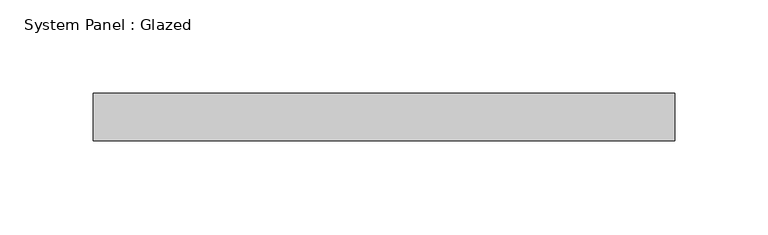
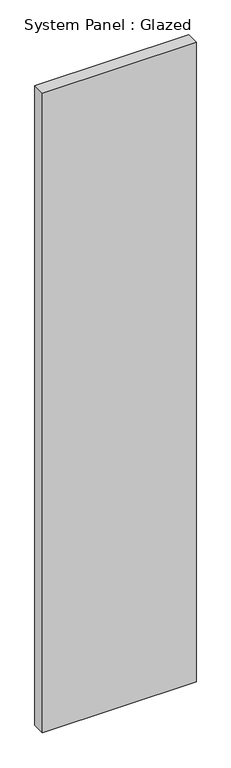
"""IFC4 building model written with IfcOpenShell, lengths in millimetres: plate geometry, System Panel : Glazed."""

from ifc_helpers import new_model, si_unit, origin, origin_with_axes, place, context, project, spatial, polyline, outline, extrude, source, transform, mapped, element, save


def system_panel_glazed_811a1c5c(model_context):
    return source(origin(), model_context, "Body", "SweptSolid", [
        extrude(outline(polyline([(155.575, 19.05), (-155.575, 19.05), (-155.575, 44.45), (155.575, 44.45), (155.575, 19.05)])), origin_with_axes(), (0.0, 0.0, 1.0), 1368.5694058),
    ])


if __name__ == "__main__":
    model = new_model("IFC4")
    model_context = context("Model", 3, world=origin())
    ifc_project = project(units=[si_unit("LENGTHUNIT", "METRE", prefix="MILLI")], contexts=[model_context])
    site = spatial("IfcSite", under=ifc_project)
    building = spatial("IfcBuilding", under=site)
    placement = place(None, origin())
    system_panel_glazed_shape = system_panel_glazed_811a1c5c(model_context)
    element("IfcPlate", 1, ObjectType="System Panel : Glazed", at=placement, inside=building, context=model_context, shape_type="MappedRepresentation", body=[
        mapped(system_panel_glazed_shape, transform((0.0, 0.0, 0.0), x_axis=(1.0, 0.0, 0.0), y_axis=(0.0, 1.0, 0.0), z_axis=(0.0, 0.0, 1.0))),
    ])
    save(model, "model.ifc")

# Revit data of these elements
# Type "System Panel : Glazed"
#   Construction Type Id = "GSP4R"
#   Analytic Construction = "1/8 in Pilkington single glazing"
#   Visual Light Transmittance = 0.9
#   Solar Heat Gain Coefficient = 0.86
#   Heat Transfer Coefficient (U) = 1.18115 BTU/(h·ft²·°F)
#   Define Thermal Properties by = 1
# Element 1 (IfcPlate, "System Panel : Glazed")
#   Materials on its faces: "Glass"
# Materials
#   "Glass": class "Glass", colour RGB 0 128 192, transparency 0.75, Description = "Soda Lime Glass", Cost = 0
